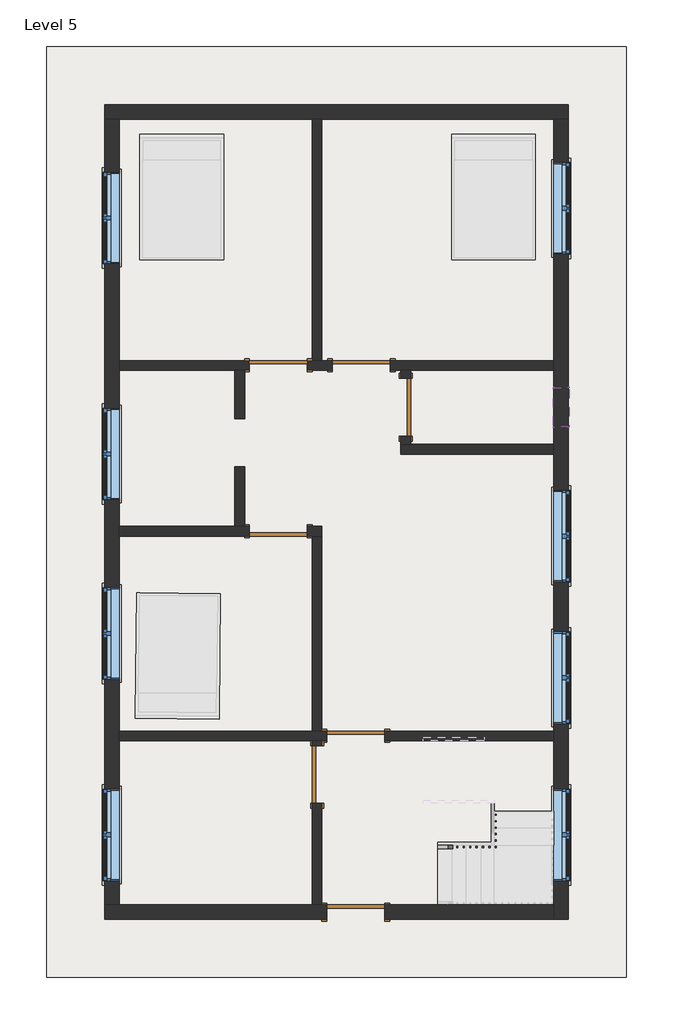
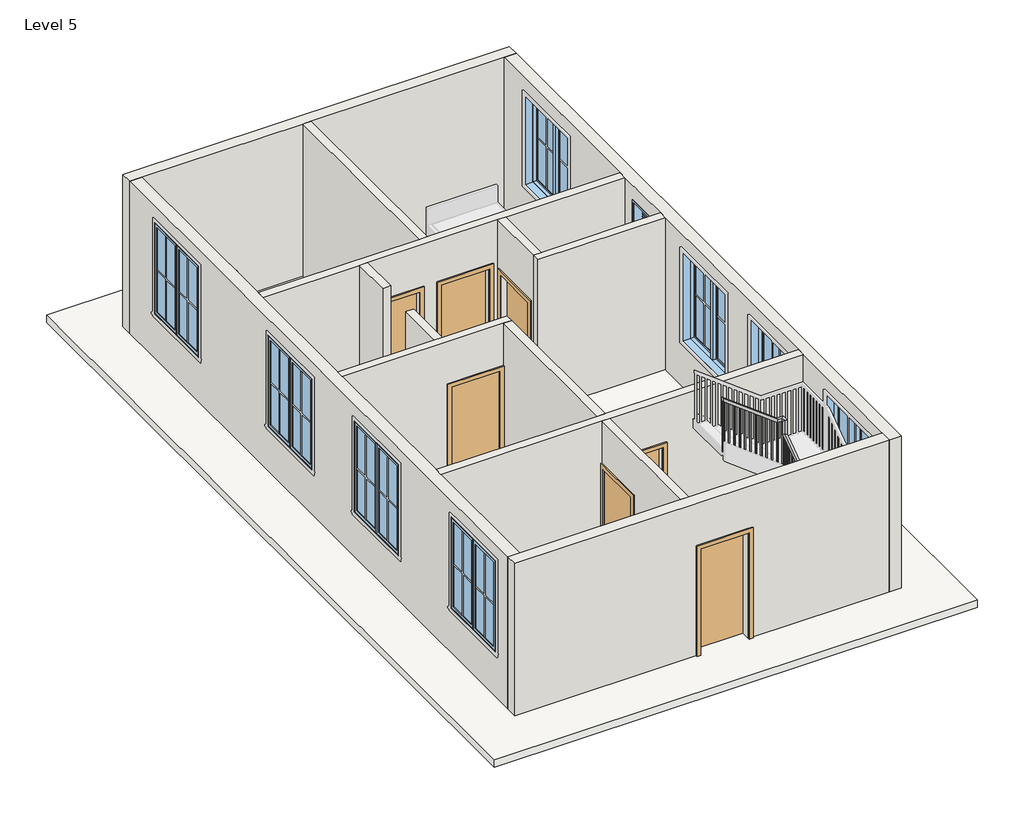
# One storey, part 1 of 2: 14 walls, 9 windows, 7 doors, 1 railing, 1 roof.
"""IFC4 building model written with IfcOpenShell, lengths in millimetres."""

from ifc_helpers import new_model, si_unit, frame, origin, place, context, project, spatial, polyline, outline, extrude, faceted_brep, transform, mapped, element, save
from components import door_2b0b55a0, door_686f89d2, door_16372e1c, door_a90ba1ad, window_9ac97e1a, window_f2d8fef0

model = new_model("IFC4")

# Units and contexts
model_context = context("Model", 3, world=origin())
ifc_project = project(units=[si_unit("LENGTHUNIT", "METRE", prefix="MILLI")], contexts=[model_context])

# Site, building, storey
site = spatial("IfcSite", under=ifc_project)
building = spatial("IfcBuilding", under=site)
storey = spatial("IfcBuildingStorey", under=building, Name="Level 5", Elevation=9601.2)

# Doors
placement = place(None, origin())
door_shape = door_2b0b55a0(model_context)
element("IfcDoor", 1, ObjectType="Single-Flush : 36\" x 80\"", at=placement, inside=storey, context=model_context, shape_type="MappedRepresentation", body=[
    mapped(door_shape, transform((-163.235885, 1707.4649429, 9601.2), x_axis=(0.0, 1.0, 0.0), y_axis=(-1.0, 0.0, 0.0), z_axis=(0.0, 0.0, 1.0))),
])
door_2_shape = door_686f89d2(model_context)
element("IfcDoor", 2, ObjectType="Single-Flush : 36\" x 84\"", at=placement, inside=storey, context=model_context, shape_type="MappedRepresentation", body=[
    mapped(door_2_shape, transform((-861.735885, 2367.8649429, 9601.2), x_axis=(-1.0, 0.0, 0.0), y_axis=(0.0, -1.0, 0.0), z_axis=(0.0, 0.0, 1.0))),
])
element("IfcDoor", 3, ObjectType="Single-Flush : 36\" x 84\"", at=placement, inside=storey, context=model_context, shape_type="MappedRepresentation", body=[
    mapped(door_2_shape, transform((-2169.835885, -248.3350571, 9601.2), x_axis=(1.0, 0.0, 0.0), y_axis=(0.0, 1.0, 0.0), z_axis=(0.0, 0.0, 1.0))),
])
element("IfcDoor", 4, ObjectType="Single-Flush : 36\" x 84\"", at=placement, inside=storey, context=model_context, shape_type="MappedRepresentation", body=[
    mapped(door_2_shape, transform((-950.635885, -3474.1350571, 9601.2), x_axis=(-1.0, 0.0, 0.0), y_axis=(0.0, -1.0, 0.0), z_axis=(0.0, 0.0, 1.0))),
])
door_3_shape = door_16372e1c(model_context)
element("IfcDoor", 5, ObjectType="Single-Flush : 36\" x 84\"", at=placement, inside=storey, context=model_context, shape_type="MappedRepresentation", body=[
    mapped(door_3_shape, transform((-2169.835885, 2367.8649429, 9601.2), x_axis=(1.0, 0.0, 0.0), y_axis=(0.0, 1.0, 0.0), z_axis=(0.0, 0.0, 1.0))),
])
element("IfcDoor", 6, ObjectType="Single-Flush : 36\" x 84\"", at=placement, inside=storey, context=model_context, shape_type="MappedRepresentation", body=[
    mapped(door_3_shape, transform((-1560.235885, -4083.7350571, 9601.2), x_axis=(0.0, 1.0, 0.0), y_axis=(-1.0, 0.0, 0.0), z_axis=(0.0, 0.0, 1.0))),
])
door_4_shape = door_a90ba1ad(model_context)
element("IfcDoor", 7, ObjectType="Single-Flush : 36\" x 84\"", at=placement, inside=storey, context=model_context, shape_type="MappedRepresentation", body=[
    mapped(door_4_shape, transform((-950.635885, -6255.4350571, 9601.2), x_axis=(-1.0, 0.0, 0.0), y_axis=(0.0, -1.0, 0.0), z_axis=(0.0, 0.0, 1.0))),
])

# Railing
element("IfcRailing", 8, ObjectType="Handrail - Rectangular", at=placement, inside=storey, context=model_context, shape_type="SolidModel", body=[
    faceted_brep([(344.764115, -5201.3350571, 10684.9333333), (344.764115, -5201.3350571, 10621.0686436), (344.764115, -5252.1350571, 10621.0686436), (344.764115, -5252.1350571, 10684.9333333), (1157.564115, -5201.3350571, 11304.2095238), (1208.364115, -5201.3350571, 11279.049596), (1208.364115, -5252.1350571, 11279.049596), (1157.564115, -5252.1350571, 11304.2095238), (1157.564115, -5201.3350571, 11586.0285714), (1208.364115, -5201.3350571, 11535.2285714), (1208.364115, -5252.1350571, 11535.2285714), (1157.564115, -5252.1350571, 11586.0285714), (1233.764115, -5201.3350571, 11586.0285714), (1233.764115, -5201.3350571, 11535.2285714), (1284.564115, -5252.1350571, 11535.2285714), (1284.564115, -5252.1350571, 11586.0285714), (1233.764115, -5125.1350571, 11586.0285714), (1233.764115, -5108.8554323, 11535.2285714), (1284.564115, -5108.8554323, 11535.2285714), (1284.564115, -5125.1350571, 11586.0285714), (1233.764115, -4566.3350571, 11985.1714286), (1233.764115, -4515.5350571, 11959.0288395), (1284.564115, -4515.5350571, 11959.0288395), (1284.564115, -4566.3350571, 11985.1714286), (1233.764115, -4566.3350571, 12266.6606061), (1233.764115, -4515.5350571, 12215.8606061), (1284.564115, -4515.5350571, 12215.8606061), (1284.564115, -4566.3350571, 12266.6606061), (1233.764115, -4490.1350571, 12266.6606061), (1233.764115, -4490.1350571, 12215.8606061), (1284.564115, -4439.3350571, 12215.8606061), (1284.564115, -4439.3350571, 12266.6606061), (1157.564115, -4490.1350571, 12266.6606061), (1140.4943334, -4490.1350571, 12215.8606061), (1140.4943334, -4439.3350571, 12215.8606061), (1157.564115, -4439.3350571, 12266.6606061), (116.164115, -4490.1350571, 13055.6), (116.164115, -4439.3350571, 13055.6), (116.164115, -4439.3350571, 12991.8683472), (116.164115, -4490.1350571, 12991.8683472)], [[[0, 1, 2, 3]], [[1, 0, 4, 5]], [[2, 1, 5, 6]], [[3, 2, 6, 7]], [[0, 3, 7, 4]], [[5, 4, 8, 9]], [[6, 5, 9, 10]], [[7, 6, 10, 11]], [[4, 7, 11, 8]], [[9, 8, 12, 13]], [[10, 9, 13, 14]], [[11, 10, 14, 15]], [[8, 11, 15, 12]], [[13, 12, 16, 17]], [[14, 13, 17, 18]], [[15, 14, 18, 19]], [[12, 15, 19, 16]], [[17, 16, 20, 21]], [[18, 17, 21, 22]], [[19, 18, 22, 23]], [[16, 19, 23, 20]], [[21, 20, 24, 25]], [[22, 21, 25, 26]], [[23, 22, 26, 27]], [[20, 23, 27, 24]], [[25, 24, 28, 29]], [[26, 25, 29, 30]], [[27, 26, 30, 31]], [[24, 27, 31, 28]], [[29, 28, 32, 33]], [[30, 29, 33, 34]], [[31, 30, 34, 35]], [[28, 31, 35, 32]], [[36, 37, 38, 39]], [[33, 32, 36, 39]], [[34, 33, 39, 38]], [[35, 34, 38, 37]], [[32, 35, 37, 36]]]),
    extrude(outline(polyline([(12979.8418321, 132.039115), (11971.8666667, 132.039115), (11971.8666667, 151.089115), (12965.4100139, 151.089115), (12979.8418321, 132.039115)])), frame((0.0, -4474.2600571, 0.0), z_axis=(0.0, 1.0, 0.0), x_axis=(0.0, 0.0, 1.0)), (0.0, 0.0, 1.0), 19.05),
    extrude(outline(polyline([(12902.8721351, 233.639115), (11971.8666667, 233.639115), (11971.8666667, 252.689115), (12888.4403169, 252.689115), (12902.8721351, 233.639115)])), frame((0.0, -4474.2600571, 0.0), z_axis=(0.0, 1.0, 0.0), x_axis=(0.0, 0.0, 1.0)), (0.0, 0.0, 1.0), 19.05),
    extrude(outline(polyline([(12825.9024382, 335.239115), (11971.8666667, 335.239115), (11971.8666667, 354.289115), (12811.47062, 354.289115), (12825.9024382, 335.239115)])), frame((0.0, -4474.2600571, 0.0), z_axis=(0.0, 1.0, 0.0), x_axis=(0.0, 0.0, 1.0)), (0.0, 0.0, 1.0), 19.05),
    extrude(outline(polyline([(12748.9327412, 436.839115), (11802.5333333, 436.839115), (11802.5333333, 455.889115), (12734.500923, 455.889115), (12748.9327412, 436.839115)])), frame((0.0, -4474.2600571, 0.0), z_axis=(0.0, 1.0, 0.0), x_axis=(0.0, 0.0, 1.0)), (0.0, 0.0, 1.0), 19.05),
    extrude(outline(polyline([(12671.9630442, 538.439115), (11802.5333333, 538.439115), (11802.5333333, 557.489115), (12657.531226, 557.489115), (12671.9630442, 538.439115)])), frame((0.0, -4474.2600571, 0.0), z_axis=(0.0, 1.0, 0.0), x_axis=(0.0, 0.0, 1.0)), (0.0, 0.0, 1.0), 19.05),
    extrude(outline(polyline([(12594.9933472, 640.039115), (11633.2, 640.039115), (11633.2, 659.089115), (12580.5615291, 659.089115), (12594.9933472, 640.039115)])), frame((0.0, -4474.2600571, 0.0), z_axis=(0.0, 1.0, 0.0), x_axis=(0.0, 0.0, 1.0)), (0.0, 0.0, 1.0), 19.05),
    extrude(outline(polyline([(12518.0236503, 741.639115), (11633.2, 741.639115), (11633.2, 760.689115), (12503.5918321, 760.689115), (12518.0236503, 741.639115)])), frame((0.0, -4474.2600571, 0.0), z_axis=(0.0, 1.0, 0.0), x_axis=(0.0, 0.0, 1.0)), (0.0, 0.0, 1.0), 19.05),
    extrude(outline(polyline([(12441.0539533, 843.239115), (11463.8666667, 843.239115), (11463.8666667, 862.289115), (12426.6221351, 862.289115), (12441.0539533, 843.239115)])), frame((0.0, -4474.2600571, 0.0), z_axis=(0.0, 1.0, 0.0), x_axis=(0.0, 0.0, 1.0)), (0.0, 0.0, 1.0), 19.05),
    extrude(outline(polyline([(12364.0842563, 944.839115), (11463.8666667, 944.839115), (11463.8666667, 963.889115), (12349.6524382, 963.889115), (12364.0842563, 944.839115)])), frame((0.0, -4474.2600571, 0.0), z_axis=(0.0, 1.0, 0.0), x_axis=(0.0, 0.0, 1.0)), (0.0, 0.0, 1.0), 19.05),
    extrude(outline(polyline([(12287.1145594, 1046.439115), (11294.5333333, 1046.439115), (11294.5333333, 1065.489115), (12272.6827412, 1065.489115), (12287.1145594, 1046.439115)])), frame((0.0, -4474.2600571, 0.0), z_axis=(0.0, 1.0, 0.0), x_axis=(0.0, 0.0, 1.0)), (0.0, 0.0, 1.0), 19.05),
    extrude(outline(polyline([(12210.1448624, 1148.039115), (11294.5333333, 1148.039115), (11294.5333333, 1167.089115), (12195.7130442, 1167.089115), (12210.1448624, 1148.039115)])), frame((0.0, -4474.2600571, 0.0), z_axis=(0.0, 1.0, 0.0), x_axis=(0.0, 0.0, 1.0)), (0.0, 0.0, 1.0), 19.05),
    extrude(outline(polyline([(1249.639115, -4525.0600571), (1249.639115, -4506.0100571), (1268.689115, -4506.0100571), (1268.689115, -4525.0600571), (1249.639115, -4525.0600571)])), frame((0.0, 0.0, 10955.8666667), z_axis=(0.0, 0.0, 1.0), x_axis=(1.0, 0.0, 0.0)), (0.0, 0.0, 1.0), 1259.9939394),
    extrude(outline(polyline([(-4607.6100571, 11893.2609823), (-4607.6100571, 10955.8666667), (-4626.6600571, 10955.8666667), (-4626.6600571, 11879.6538395), (-4607.6100571, 11893.2609823)])), frame((1249.639115, 0.0, 0.0), z_axis=(1.0, 0.0, 0.0), x_axis=(0.0, 1.0, 0.0)), (0.0, 0.0, 1.0), 19.05),
    extrude(outline(polyline([(-4709.2100571, 11820.6895538), (-4709.2100571, 10786.5333333), (-4728.2600571, 10786.5333333), (-4728.2600571, 11807.0824109), (-4709.2100571, 11820.6895538)])), frame((1249.639115, 0.0, 0.0), z_axis=(1.0, 0.0, 0.0), x_axis=(0.0, 1.0, 0.0)), (0.0, 0.0, 1.0), 19.05),
    extrude(outline(polyline([(-4810.8100571, 11748.1181252), (-4810.8100571, 10786.5333333), (-4829.8600571, 10786.5333333), (-4829.8600571, 11734.5109823), (-4810.8100571, 11748.1181252)])), frame((1249.639115, 0.0, 0.0), z_axis=(1.0, 0.0, 0.0), x_axis=(0.0, 1.0, 0.0)), (0.0, 0.0, 1.0), 19.05),
    extrude(outline(polyline([(-4912.4100571, 11675.5466966), (-4912.4100571, 10786.5333333), (-4931.4600571, 10786.5333333), (-4931.4600571, 11661.9395538), (-4912.4100571, 11675.5466966)])), frame((1249.639115, 0.0, 0.0), z_axis=(1.0, 0.0, 0.0), x_axis=(0.0, 1.0, 0.0)), (0.0, 0.0, 1.0), 19.05),
    extrude(outline(polyline([(-5014.0100571, 11602.9752681), (-5014.0100571, 10617.2), (-5033.0600571, 10617.2), (-5033.0600571, 11589.3681252), (-5014.0100571, 11602.9752681)])), frame((1249.639115, 0.0, 0.0), z_axis=(1.0, 0.0, 0.0), x_axis=(0.0, 1.0, 0.0)), (0.0, 0.0, 1.0), 19.05),
    extrude(outline(polyline([(-5115.6100571, 11530.4038395), (-5115.6100571, 10617.2), (-5134.6600571, 10617.2), (-5134.6600571, 11516.7966966), (-5115.6100571, 11530.4038395)])), frame((1249.639115, 0.0, 0.0), z_axis=(1.0, 0.0, 0.0), x_axis=(0.0, 1.0, 0.0)), (0.0, 0.0, 1.0), 19.05),
    extrude(outline(polyline([(11233.0876912, 1148.039115), (10278.5333333, 1148.039115), (10278.5333333, 1167.089115), (11247.6019769, 1167.089115), (11233.0876912, 1148.039115)])), frame((0.0, -5236.2600571, 0.0), z_axis=(0.0, 1.0, 0.0), x_axis=(0.0, 0.0, 1.0)), (0.0, 0.0, 1.0), 19.05),
    extrude(outline(polyline([(11155.6781674, 1046.439115), (10278.5333333, 1046.439115), (10278.5333333, 1065.489115), (11170.1924531, 1065.489115), (11155.6781674, 1046.439115)])), frame((0.0, -5236.2600571, 0.0), z_axis=(0.0, 1.0, 0.0), x_axis=(0.0, 0.0, 1.0)), (0.0, 0.0, 1.0), 19.05),
    extrude(outline(polyline([(11078.2686436, 944.839115), (10109.2, 944.839115), (10109.2, 963.889115), (11092.7829293, 963.889115), (11078.2686436, 944.839115)])), frame((0.0, -5236.2600571, 0.0), z_axis=(0.0, 1.0, 0.0), x_axis=(0.0, 0.0, 1.0)), (0.0, 0.0, 1.0), 19.05),
    extrude(outline(polyline([(11000.8591198, 843.239115), (10109.2, 843.239115), (10109.2, 862.289115), (11015.3734055, 862.289115), (11000.8591198, 843.239115)])), frame((0.0, -5236.2600571, 0.0), z_axis=(0.0, 1.0, 0.0), x_axis=(0.0, 0.0, 1.0)), (0.0, 0.0, 1.0), 19.05),
    extrude(outline(polyline([(10923.449596, 741.639115), (9939.8666667, 741.639115), (9939.8666667, 760.689115), (10937.9638817, 760.689115), (10923.449596, 741.639115)])), frame((0.0, -5236.2600571, 0.0), z_axis=(0.0, 1.0, 0.0), x_axis=(0.0, 0.0, 1.0)), (0.0, 0.0, 1.0), 19.05),
    extrude(outline(polyline([(10846.0400722, 640.039115), (9939.8666667, 640.039115), (9939.8666667, 659.089115), (10860.5543579, 659.089115), (10846.0400722, 640.039115)])), frame((0.0, -5236.2600571, 0.0), z_axis=(0.0, 1.0, 0.0), x_axis=(0.0, 0.0, 1.0)), (0.0, 0.0, 1.0), 19.05),
    extrude(outline(polyline([(10768.6305484, 538.439115), (9770.5333333, 538.439115), (9770.5333333, 557.489115), (10783.1448341, 557.489115), (10768.6305484, 538.439115)])), frame((0.0, -5236.2600571, 0.0), z_axis=(0.0, 1.0, 0.0), x_axis=(0.0, 0.0, 1.0)), (0.0, 0.0, 1.0), 19.05),
    extrude(outline(polyline([(10691.2210246, 436.839115), (9770.5333333, 436.839115), (9770.5333333, 455.889115), (10705.7353103, 455.889115), (10691.2210246, 436.839115)])), frame((0.0, -5236.2600571, 0.0), z_axis=(0.0, 1.0, 0.0), x_axis=(0.0, 0.0, 1.0)), (0.0, 0.0, 1.0), 19.05),
    extrude(outline(polyline([(1249.639115, -4474.2600571), (1249.639115, -4455.2100571), (1268.689115, -4455.2100571), (1268.689115, -4474.2600571), (1249.639115, -4474.2600571)])), frame((0.0, 0.0, 11125.2), z_axis=(0.0, 0.0, 1.0), x_axis=(1.0, 0.0, 0.0)), (0.0, 0.0, 1.0), 1090.6606061),
    extrude(outline(polyline([(1249.639115, -5217.2100571), (1268.689115, -5217.2100571), (1268.689115, -5236.2600571), (1249.639115, -5236.2600571), (1249.639115, -5217.2100571)])), frame((0.0, 0.0, 10447.8666667), z_axis=(0.0, 0.0, 1.0), x_axis=(1.0, 0.0, 0.0)), (0.0, 0.0, 1.0), 1087.3619048),
    extrude(outline(polyline([(12991.8683472, 116.164115), (11971.8666667, 116.164115), (11971.8666667, 135.214115), (12977.4365291, 135.214115), (12991.8683472, 116.164115)])), frame((0.0, -4474.2600571, 0.0), z_axis=(0.0, 1.0, 0.0), x_axis=(0.0, 0.0, 1.0)), (0.0, 0.0, 1.0), 19.05),
    extrude(outline(polyline([(10621.0686436, 344.764115), (9770.5333333, 344.764115), (9770.5333333, 363.814115), (10635.5829293, 363.814115), (10621.0686436, 344.764115)])), frame((0.0, -5236.2600571, 0.0), z_axis=(0.0, 1.0, 0.0), x_axis=(0.0, 0.0, 1.0)), (0.0, 0.0, 1.0), 19.05),
])

# Roof
element("IfcRoof", 9, ObjectType="ROOF 6\"", at=placement, inside=storey, context=model_context, shape_type="SweptSolid", body=[
    extrude(outline(polyline([(-5827.435885, 7397.0649429), (3316.564115, 7397.0649429), (3316.564115, -7284.1350571), (-5827.435885, -7284.1350571), (-5827.435885, 7397.0649429)])), frame((0.0, 0.0, 9448.8), z_axis=(0.0, 0.0, 1.0), x_axis=(1.0, 0.0, 0.0)), (0.0, 0.0, 1.0), 152.4),
])

# Walls
element("IfcWall", 10, ObjectType="WALL 6\"", at=placement, inside=storey, context=model_context, shape_type="SweptSolid", body=[
    extrude(outline(polyline([(-1636.435885, 2444.0649429), (-1636.435885, 6254.0649429), (-1484.035885, 6254.0649429), (-1484.035885, 2444.0649429), (-1636.435885, 2444.0649429)])), frame((0.0, 0.0, 9601.2), z_axis=(0.0, 0.0, 1.0), x_axis=(1.0, 0.0, 0.0)), (0.0, 0.0, 1.0), 3048.0),
])
element("IfcWall", 11, ObjectType="WALL 6\"", at=placement, inside=storey, context=model_context, shape_type="Brep", body=[
    faceted_brep([(-1318.935885, 2444.0649429, 9601.2), (-1484.035885, 2444.0649429, 9601.2), (-1636.435885, 2444.0649429, 9601.2), (-1712.635885, 2444.0649429, 9601.2), (-1712.635885, 2444.0649429, 11734.8), (-2627.035885, 2444.0649429, 11734.8), (-2627.035885, 2444.0649429, 9601.2), (-4684.435885, 2444.0649429, 9601.2), (-4684.435885, 2444.0649429, 12649.2), (-1636.435885, 2444.0649429, 12649.2), (-1484.035885, 2444.0649429, 12649.2), (2173.564115, 2444.0649429, 12649.2), (2173.564115, 2444.0649429, 9601.2), (-404.535885, 2444.0649429, 9601.2), (-404.535885, 2444.0649429, 11734.8), (-1318.935885, 2444.0649429, 11734.8), (-1712.635885, 2291.6649429, 11734.8), (-1712.635885, 2291.6649429, 9601.2), (-1318.935885, 2291.6649429, 9601.2), (-1318.935885, 2291.6649429, 11734.8), (-404.535885, 2291.6649429, 11734.8), (-404.535885, 2291.6649429, 9601.2), (-239.435885, 2291.6649429, 9601.2), (-87.035885, 2291.6649429, 9601.2), (2173.564115, 2291.6649429, 9601.2), (2173.564115, 2291.6649429, 12649.2), (-87.035885, 2291.6649429, 12649.2), (-239.435885, 2291.6649429, 12649.2), (-2703.235885, 2291.6649429, 12649.2), (-2855.635885, 2291.6649429, 12649.2), (-4684.435885, 2291.6649429, 12649.2), (-4684.435885, 2291.6649429, 9601.2), (-2855.635885, 2291.6649429, 9601.2), (-2703.235885, 2291.6649429, 9601.2), (-2627.035885, 2291.6649429, 9601.2), (-2627.035885, 2291.6649429, 11734.8)], [[[0, 1, 2, 3, 4, 5, 6, 7, 8, 9, 10, 11, 12, 13, 14, 15]], [[16, 17, 18, 19, 20, 21, 22, 23, 24, 25, 26, 27, 28, 29, 30, 31, 32, 33, 34, 35]], [[13, 12, 24, 23, 22, 21]], [[18, 17, 3, 2, 1, 0]], [[34, 33, 32, 31, 7, 6]], [[12, 11, 25, 24]], [[8, 7, 31, 30]], [[19, 18, 0, 15]], [[20, 19, 15, 14]], [[21, 20, 14, 13]], [[4, 3, 17, 16]], [[5, 4, 16, 35]], [[6, 5, 35, 34]], [[11, 10, 9, 8, 30, 29, 28, 27, 26, 25]]]),
])
element("IfcWall", 12, ObjectType="WALL 6\"", at=placement, inside=storey, context=model_context, shape_type="SweptSolid", body=[
    extrude(outline(polyline([(-2855.635885, 1529.6649429), (-2855.635885, 2291.6649429), (-2703.235885, 2291.6649429), (-2703.235885, 1529.6649429), (-2855.635885, 1529.6649429)])), frame((0.0, 0.0, 9601.2), z_axis=(0.0, 0.0, 1.0), x_axis=(1.0, 0.0, 0.0)), (0.0, 0.0, 1.0), 3048.0),
])
element("IfcWall", 13, ObjectType="WALL 6\"", at=placement, inside=storey, context=model_context, shape_type="Brep", body=[
    faceted_brep([(-1712.635885, -324.5350571, 11734.8), (-1712.635885, -324.5350571, 9601.2), (-1636.435885, -324.5350571, 9601.2), (-1484.035885, -324.5350571, 9601.2), (-1484.035885, -324.5350571, 12649.2), (-1636.435885, -324.5350571, 12649.2), (-4684.435885, -324.5350571, 12649.2), (-4684.435885, -324.5350571, 9601.2), (-2627.035885, -324.5350571, 9601.2), (-2627.035885, -324.5350571, 11734.8), (-1484.035885, -172.1350571, 9601.2), (-1712.635885, -172.1350571, 9601.2), (-1712.635885, -172.1350571, 11734.8), (-2627.035885, -172.1350571, 11734.8), (-2627.035885, -172.1350571, 9601.2), (-2703.235885, -172.1350571, 9601.2), (-2855.635885, -172.1350571, 9601.2), (-4684.435885, -172.1350571, 9601.2), (-4684.435885, -172.1350571, 12649.2), (-2855.635885, -172.1350571, 12649.2), (-2703.235885, -172.1350571, 12649.2), (-1484.035885, -172.1350571, 12649.2)], [[[0, 1, 2, 3, 4, 5, 6, 7, 8, 9]], [[10, 11, 12, 13, 14, 15, 16, 17, 18, 19, 20, 21]], [[8, 7, 17, 16, 15, 14]], [[3, 2, 1, 11, 10]], [[7, 6, 18, 17]], [[4, 3, 10, 21]], [[12, 11, 1, 0]], [[13, 12, 0, 9]], [[14, 13, 9, 8]], [[6, 5, 4, 21, 20, 19, 18]]]),
])
element("IfcWall", 14, ObjectType="WALL 6\"", at=placement, inside=storey, context=model_context, shape_type="SweptSolid", body=[
    extrude(outline(polyline([(-1636.435885, -3397.9350571), (-1636.435885, -324.5350571), (-1484.035885, -324.5350571), (-1484.035885, -3397.9350571), (-1636.435885, -3397.9350571)])), frame((0.0, 0.0, 9601.2), z_axis=(0.0, 0.0, 1.0), x_axis=(1.0, 0.0, 0.0)), (0.0, 0.0, 1.0), 3048.0),
])
element("IfcWall", 15, ObjectType="WALL 6\"", at=placement, inside=storey, context=model_context, shape_type="Brep", body=[
    faceted_brep([(-4684.435885, -3550.3350571, 9601.2), (-1636.435885, -3550.3350571, 9601.2), (-1484.035885, -3550.3350571, 9601.2), (-1407.835885, -3550.3350571, 9601.2), (-1407.835885, -3550.3350571, 11734.8), (-493.435885, -3550.3350571, 11734.8), (-493.435885, -3550.3350571, 9601.2), (2173.564115, -3550.3350571, 9601.2), (2173.564115, -3550.3350571, 12649.2), (-1484.035885, -3550.3350571, 12649.2), (-1636.435885, -3550.3350571, 12649.2), (-4684.435885, -3550.3350571, 12649.2), (-1407.835885, -3397.9350571, 11734.8), (-1407.835885, -3397.9350571, 9601.2), (-1484.035885, -3397.9350571, 9601.2), (-1636.435885, -3397.9350571, 9601.2), (-4684.435885, -3397.9350571, 9601.2), (-4684.435885, -3397.9350571, 12649.2), (-1636.435885, -3397.9350571, 12649.2), (-1484.035885, -3397.9350571, 12649.2), (2173.564115, -3397.9350571, 12649.2), (2173.564115, -3397.9350571, 9601.2), (-493.435885, -3397.9350571, 9601.2), (-493.435885, -3397.9350571, 11734.8)], [[[0, 1, 2, 3, 4, 5, 6, 7, 8, 9, 10, 11]], [[12, 13, 14, 15, 16, 17, 18, 19, 20, 21, 22, 23]], [[22, 21, 7, 6]], [[16, 15, 14, 13, 3, 2, 1, 0]], [[8, 7, 21, 20]], [[0, 11, 17, 16]], [[4, 3, 13, 12]], [[5, 4, 12, 23]], [[6, 5, 23, 22]], [[11, 10, 9, 8, 20, 19, 18, 17]]]),
])
element("IfcWall", 16, ObjectType="WALL 6\"", at=placement, inside=storey, context=model_context, shape_type="SweptSolid", body=[
    extrude(outline(polyline([(-3550.3350571, 9601.2), (-3626.5350571, 9601.2), (-3626.5350571, 11734.8), (-4540.9350571, 11734.8), (-4540.9350571, 9601.2), (-6141.1350571, 9601.2), (-6141.1350571, 12649.2), (-3550.3350571, 12649.2), (-3550.3350571, 9601.2)])), frame((-1636.435885, 0.0, 0.0), z_axis=(1.0, 0.0, 0.0), x_axis=(0.0, 1.0, 0.0)), (0.0, 0.0, 1.0), 152.4),
])
element("IfcWall", 17, ObjectType="WALL 6\"", at=placement, inside=storey, context=model_context, shape_type="Brep", body=[
    faceted_brep([(2173.564115, 1123.2649429, 9601.2), (-87.035885, 1123.2649429, 9601.2), (-239.435885, 1123.2649429, 9601.2), (-239.435885, 1123.2649429, 12649.2), (-87.035885, 1123.2649429, 12649.2), (2173.564115, 1123.2649429, 12649.2), (2173.564115, 970.8649429, 9601.2), (2173.564115, 970.8649429, 12649.2), (-239.435885, 970.8649429, 12649.2), (-239.435885, 970.8649429, 9601.2)], [[[0, 1, 2, 3, 4, 5]], [[6, 7, 8, 9]], [[2, 1, 0, 6, 9]], [[0, 5, 7, 6]], [[3, 2, 9, 8]], [[5, 4, 3, 8, 7]]]),
])
element("IfcWall", 18, ObjectType="WALL 6\"", at=placement, inside=storey, context=model_context, shape_type="SweptSolid", body=[
    extrude(outline(polyline([(2291.6649429, 9601.2), (2164.6649429, 9601.2), (2164.6649429, 11633.2), (1250.2649429, 11633.2), (1250.2649429, 9601.2), (1123.2649429, 9601.2), (1123.2649429, 12649.2), (2291.6649429, 12649.2), (2291.6649429, 9601.2)])), frame((-239.435885, 0.0, 0.0), z_axis=(1.0, 0.0, 0.0), x_axis=(0.0, 1.0, 0.0)), (0.0, 0.0, 1.0), 152.4),
])
element("IfcWall", 19, ObjectType="WALL 6\"", at=placement, inside=storey, context=model_context, shape_type="SweptSolid", body=[
    extrude(outline(polyline([(-2855.635885, -172.1350571), (-2855.635885, 767.6649429), (-2703.235885, 767.6649429), (-2703.235885, -172.1350571), (-2855.635885, -172.1350571)])), frame((0.0, 0.0, 9601.2), z_axis=(0.0, 0.0, 1.0), x_axis=(1.0, 0.0, 0.0)), (0.0, 0.0, 1.0), 3048.0),
])
element("IfcWall", 20, ObjectType="WALL 9\"", at=placement, inside=storey, context=model_context, shape_type="Brep", body=[
    faceted_brep([(-4913.035885, 6254.0649429, 9601.2), (-4684.435885, 6254.0649429, 9601.2), (-1636.435885, 6254.0649429, 9601.2), (-1484.035885, 6254.0649429, 9601.2), (2173.564115, 6254.0649429, 9601.2), (2402.164115, 6254.0649429, 9601.2), (2402.164115, 6254.0649429, 12649.2), (2173.564115, 6254.0649429, 12649.2), (-1484.035885, 6254.0649429, 12649.2), (-1636.435885, 6254.0649429, 12649.2), (-4684.435885, 6254.0649429, 12649.2), (-4913.035885, 6254.0649429, 12649.2), (-4913.035885, 6482.6649429, 9601.2), (-4913.035885, 6482.6649429, 12649.2), (2402.164115, 6482.6649429, 12649.2), (2402.164115, 6482.6649429, 9601.2)], [[[0, 1, 2, 3, 4, 5, 6, 7, 8, 9, 10, 11]], [[12, 13, 14, 15]], [[5, 4, 3, 2, 1, 0, 12, 15]], [[6, 5, 15, 14]], [[0, 11, 13, 12]], [[11, 10, 9, 8, 7, 6, 14, 13]]]),
])
element("IfcWall", 21, ObjectType="WALL 9\"", at=placement, inside=storey, context=model_context, shape_type="Brep", body=[
    faceted_brep([(2173.564115, 6254.0649429, 9601.2), (2173.564115, 2444.0649429, 9601.2), (2173.564115, 2291.6649429, 9601.2), (2173.564115, 1123.2649429, 9601.2), (2173.564115, 970.8649429, 9601.2), (2173.564115, -3397.9350571, 9601.2), (2173.564115, -3550.3350571, 9601.2), (2173.564115, -6141.1350571, 9601.2), (2173.564115, -6369.7350571, 9601.2), (2173.564115, -6369.7350571, 12649.2), (2173.564115, -6141.1350571, 12649.2), (2173.564115, -3550.3350571, 12649.2), (2173.564115, -3397.9350571, 12649.2), (2173.564115, 970.8649429, 12649.2), (2173.564115, 1123.2649429, 12649.2), (2173.564115, 2291.6649429, 12649.2), (2173.564115, 2444.0649429, 12649.2), (2173.564115, 6254.0649429, 12649.2), (2173.564115, -5760.1350571, 12344.4), (2173.564115, -5760.1350571, 10515.6), (2173.564115, -4312.3350571, 10515.6), (2173.564115, -4312.3350571, 12344.4), (2173.564115, -3283.6350571, 12344.4), (2173.564115, -3283.6350571, 10515.6), (2173.564115, -1835.8350571, 10515.6), (2173.564115, -1835.8350571, 12344.4), (2173.564115, -1048.4350571, 12344.4), (2173.564115, -1048.4350571, 10515.6), (2173.564115, 399.3649429, 10515.6), (2173.564115, 399.3649429, 12344.4), (2173.564115, 4120.4649429, 12344.4), (2173.564115, 4120.4649429, 10515.6), (2173.564115, 5568.2649429, 10515.6), (2173.564115, 5568.2649429, 12344.4), (2173.564115, 2012.2649429, 12344.4), (2173.564115, 1402.6649429, 12344.4), (2173.564115, 1402.6649429, 11734.8), (2173.564115, 2012.2649429, 11734.8), (2402.164115, 6254.0649429, 9601.2), (2402.164115, 6254.0649429, 12649.2), (2402.164115, -6369.7350571, 12649.2), (2402.164115, -6369.7350571, 9601.2), (2402.164115, -5760.1350571, 12344.4), (2402.164115, -4312.3350571, 12344.4), (2402.164115, -4312.3350571, 10515.6), (2402.164115, -5760.1350571, 10515.6), (2402.164115, -3283.6350571, 12344.4), (2402.164115, -1835.8350571, 12344.4), (2402.164115, -1835.8350571, 10515.6), (2402.164115, -3283.6350571, 10515.6), (2402.164115, -1048.4350571, 12344.4), (2402.164115, 399.3649429, 12344.4), (2402.164115, 399.3649429, 10515.6), (2402.164115, -1048.4350571, 10515.6), (2402.164115, 4120.4649429, 12344.4), (2402.164115, 5568.2649429, 12344.4), (2402.164115, 5568.2649429, 10515.6), (2402.164115, 4120.4649429, 10515.6), (2402.164115, 2012.2649429, 12344.4), (2402.164115, 2012.2649429, 11734.8), (2402.164115, 1402.6649429, 11734.8), (2402.164115, 1402.6649429, 12344.4)], [[[0, 1, 2, 3, 4, 5, 6, 7, 8, 9, 10, 11, 12, 13, 14, 15, 16, 17], [18, 19, 20, 21], [22, 23, 24, 25], [26, 27, 28, 29], [30, 31, 32, 33], [34, 35, 36, 37]], [[38, 39, 40, 41], [42, 43, 44, 45], [46, 47, 48, 49], [50, 51, 52, 53], [54, 55, 56, 57], [58, 59, 60, 61]], [[8, 7, 6, 5, 4, 3, 2, 1, 0, 38, 41]], [[0, 17, 39, 38]], [[9, 8, 41, 40]], [[19, 18, 42, 45]], [[20, 19, 45, 44]], [[21, 20, 44, 43]], [[18, 21, 43, 42]], [[23, 22, 46, 49]], [[24, 23, 49, 48]], [[25, 24, 48, 47]], [[22, 25, 47, 46]], [[27, 26, 50, 53]], [[28, 27, 53, 52]], [[29, 28, 52, 51]], [[26, 29, 51, 50]], [[31, 30, 54, 57]], [[32, 31, 57, 56]], [[33, 32, 56, 55]], [[30, 33, 55, 54]], [[59, 58, 34, 37]], [[60, 59, 37, 36]], [[61, 60, 36, 35]], [[58, 61, 35, 34]], [[17, 16, 15, 14, 13, 12, 11, 10, 9, 40, 39]]]),
])
element("IfcWall", 22, ObjectType="WALL 9\"", at=placement, inside=storey, context=model_context, shape_type="Brep", body=[
    faceted_brep([(-1407.835885, -6141.1350571, 11734.8), (-1407.835885, -6141.1350571, 9601.2), (-1484.035885, -6141.1350571, 9601.2), (-1636.435885, -6141.1350571, 9601.2), (-4684.435885, -6141.1350571, 9601.2), (-4913.035885, -6141.1350571, 9601.2), (-4913.035885, -6141.1350571, 12649.2), (-4684.435885, -6141.1350571, 12649.2), (-1636.435885, -6141.1350571, 12649.2), (-1484.035885, -6141.1350571, 12649.2), (2173.564115, -6141.1350571, 12649.2), (2173.564115, -6141.1350571, 9601.2), (-493.435885, -6141.1350571, 9601.2), (-493.435885, -6141.1350571, 11734.8), (-4913.035885, -6369.7350571, 9601.2), (-1407.835885, -6369.7350571, 9601.2), (-1407.835885, -6369.7350571, 11734.8), (-493.435885, -6369.7350571, 11734.8), (-493.435885, -6369.7350571, 9601.2), (2173.564115, -6369.7350571, 9601.2), (2173.564115, -6369.7350571, 12649.2), (-4913.035885, -6369.7350571, 12649.2)], [[[0, 1, 2, 3, 4, 5, 6, 7, 8, 9, 10, 11, 12, 13]], [[14, 15, 16, 17, 18, 19, 20, 21]], [[12, 11, 19, 18]], [[5, 4, 3, 2, 1, 15, 14]], [[11, 10, 20, 19]], [[6, 5, 14, 21]], [[16, 15, 1, 0]], [[17, 16, 0, 13]], [[18, 17, 13, 12]], [[10, 9, 8, 7, 6, 21, 20]]]),
])
element("IfcWall", 23, ObjectType="WALL 9\"", at=placement, inside=storey, context=model_context, shape_type="Brep", body=[
    faceted_brep([(-4684.435885, -6141.1350571, 9601.2), (-4684.435885, -3550.3350571, 9601.2), (-4684.435885, -3397.9350571, 9601.2), (-4684.435885, -324.5350571, 9601.2), (-4684.435885, -172.1350571, 9601.2), (-4684.435885, 2291.6649429, 9601.2), (-4684.435885, 2444.0649429, 9601.2), (-4684.435885, 6254.0649429, 9601.2), (-4684.435885, 6254.0649429, 12649.2), (-4684.435885, 2444.0649429, 12649.2), (-4684.435885, 2291.6649429, 12649.2), (-4684.435885, -172.1350571, 12649.2), (-4684.435885, -324.5350571, 12649.2), (-4684.435885, -3397.9350571, 12649.2), (-4684.435885, -3550.3350571, 12649.2), (-4684.435885, -6141.1350571, 12649.2), (-4684.435885, -4312.3350571, 12344.4), (-4684.435885, -4312.3350571, 10515.6), (-4684.435885, -5760.1350571, 10515.6), (-4684.435885, -5760.1350571, 12344.4), (-4684.435885, -1137.3350571, 12344.4), (-4684.435885, -1137.3350571, 10515.6), (-4684.435885, -2585.1350571, 10515.6), (-4684.435885, -2585.1350571, 12344.4), (-4684.435885, 1694.7649429, 12344.4), (-4684.435885, 1694.7649429, 10515.6), (-4684.435885, 246.9649429, 10515.6), (-4684.435885, 246.9649429, 12344.4), (-4684.435885, 5415.8649429, 12344.4), (-4684.435885, 5415.8649429, 10515.6), (-4684.435885, 3968.0649429, 10515.6), (-4684.435885, 3968.0649429, 12344.4), (-4913.035885, -6141.1350571, 9601.2), (-4913.035885, -6141.1350571, 12649.2), (-4913.035885, 6254.0649429, 12649.2), (-4913.035885, 6254.0649429, 9601.2), (-4913.035885, -4312.3350571, 12344.4), (-4913.035885, -5760.1350571, 12344.4), (-4913.035885, -5760.1350571, 10515.6), (-4913.035885, -4312.3350571, 10515.6), (-4913.035885, -1137.3350571, 12344.4), (-4913.035885, -2585.1350571, 12344.4), (-4913.035885, -2585.1350571, 10515.6), (-4913.035885, -1137.3350571, 10515.6), (-4913.035885, 1694.7649429, 12344.4), (-4913.035885, 246.9649429, 12344.4), (-4913.035885, 246.9649429, 10515.6), (-4913.035885, 1694.7649429, 10515.6), (-4913.035885, 5415.8649429, 12344.4), (-4913.035885, 3968.0649429, 12344.4), (-4913.035885, 3968.0649429, 10515.6), (-4913.035885, 5415.8649429, 10515.6)], [[[0, 1, 2, 3, 4, 5, 6, 7, 8, 9, 10, 11, 12, 13, 14, 15], [16, 17, 18, 19], [20, 21, 22, 23], [24, 25, 26, 27], [28, 29, 30, 31]], [[32, 33, 34, 35], [36, 37, 38, 39], [40, 41, 42, 43], [44, 45, 46, 47], [48, 49, 50, 51]], [[7, 6, 5, 4, 3, 2, 1, 0, 32, 35]], [[8, 7, 35, 34]], [[0, 15, 33, 32]], [[17, 16, 36, 39]], [[18, 17, 39, 38]], [[19, 18, 38, 37]], [[16, 19, 37, 36]], [[21, 20, 40, 43]], [[22, 21, 43, 42]], [[23, 22, 42, 41]], [[20, 23, 41, 40]], [[25, 24, 44, 47]], [[26, 25, 47, 46]], [[27, 26, 46, 45]], [[24, 27, 45, 44]], [[29, 28, 48, 51]], [[30, 29, 51, 50]], [[31, 30, 50, 49]], [[28, 31, 49, 48]], [[15, 14, 13, 12, 11, 10, 9, 8, 34, 33]]]),
])

# Windows
window_shape = window_9ac97e1a(model_context)
element("IfcWindow", 24, ObjectType="Window-Casement-Double : 57\" x 72\"", at=placement, inside=storey, context=model_context, shape_type="MappedRepresentation", body=[
    mapped(window_shape, transform((-4798.735885, -5036.2350571, 9601.2), x_axis=(0.0, 1.0, 0.0), y_axis=(-1.0, 0.0, 0.0), z_axis=(0.0, 0.0, 1.0))),
])
element("IfcWindow", 25, ObjectType="Window-Casement-Double : 57\" x 72\"", at=placement, inside=storey, context=model_context, shape_type="MappedRepresentation", body=[
    mapped(window_shape, transform((2287.864115, -5036.2350571, 9601.2), x_axis=(0.0, -1.0, 0.0), y_axis=(1.0, 0.0, 0.0), z_axis=(0.0, 0.0, 1.0))),
])
element("IfcWindow", 26, ObjectType="Window-Casement-Double : 57\" x 72\"", at=placement, inside=storey, context=model_context, shape_type="MappedRepresentation", body=[
    mapped(window_shape, transform((2287.864115, -2559.7350571, 9601.2), x_axis=(0.0, -1.0, 0.0), y_axis=(1.0, 0.0, 0.0), z_axis=(0.0, 0.0, 1.0))),
])
element("IfcWindow", 27, ObjectType="Window-Casement-Double : 57\" x 72\"", at=placement, inside=storey, context=model_context, shape_type="MappedRepresentation", body=[
    mapped(window_shape, transform((2287.864115, -324.5350571, 9601.2), x_axis=(0.0, -1.0, 0.0), y_axis=(1.0, 0.0, 0.0), z_axis=(0.0, 0.0, 1.0))),
])
element("IfcWindow", 28, ObjectType="Window-Casement-Double : 57\" x 72\"", at=placement, inside=storey, context=model_context, shape_type="MappedRepresentation", body=[
    mapped(window_shape, transform((-4798.735885, -1861.2350571, 9601.2), x_axis=(0.0, 1.0, 0.0), y_axis=(-1.0, 0.0, 0.0), z_axis=(0.0, 0.0, 1.0))),
])
element("IfcWindow", 29, ObjectType="Window-Casement-Double : 57\" x 72\"", at=placement, inside=storey, context=model_context, shape_type="MappedRepresentation", body=[
    mapped(window_shape, transform((-4798.735885, 970.8649429, 9601.2), x_axis=(0.0, 1.0, 0.0), y_axis=(-1.0, 0.0, 0.0), z_axis=(0.0, 0.0, 1.0))),
])
element("IfcWindow", 30, ObjectType="Window-Casement-Double : 57\" x 72\"", at=placement, inside=storey, context=model_context, shape_type="MappedRepresentation", body=[
    mapped(window_shape, transform((-4798.735885, 4691.9649429, 9601.2), x_axis=(0.0, 1.0, 0.0), y_axis=(-1.0, 0.0, 0.0), z_axis=(0.0, 0.0, 1.0))),
])
element("IfcWindow", 31, ObjectType="Window-Casement-Double : 57\" x 72\"", at=placement, inside=storey, context=model_context, shape_type="MappedRepresentation", body=[
    mapped(window_shape, transform((2287.864115, 4844.3649429, 9601.2), x_axis=(0.0, -1.0, 0.0), y_axis=(1.0, 0.0, 0.0), z_axis=(0.0, 0.0, 1.0))),
])
window_2_shape = window_f2d8fef0(model_context)
element("IfcWindow", 32, ObjectType="Window-Louvers : 24\" x 24\"", at=placement, inside=storey, context=model_context, shape_type="MappedRepresentation", body=[
    mapped(window_2_shape, transform((2294.214115, 1707.4649429, 10820.4), x_axis=(0.0, -1.0, 0.0), y_axis=(1.0, 0.0, 0.0), z_axis=(0.0, 0.0, 1.0))),
])

save(model, "model.ifc")

# Revit data of these elements
# Type "Single-Flush : 36\" x 80\""
#   Type Mark = "6"
#   Construction Type Id = "MDOOR"
#   Assembly Code = "C1020"
#   Analytic Construction = "Metal"
#   Thickness = 0' - 2"
#   Heat Transfer Coefficient (U) = 0.651978 BTU/(h·ft²·°F)
#   Height = 6' - 8"
#   Trim Projection Ext = 0' - 1"
#   Trim Projection Int = 0' - 1"
#   Trim Width = 0' - 3"
#   Width = 3' - 0"
#   Define Thermal Properties by = 1
#   Define Thermal Properties by = 1
#   Door Material = Door - Panel
#   Frame Material = Door - Frame
#   Visual Light Transmittance = 0
#   Solar Heat Gain Coefficient = 0
#   Function = (empty or 0)
#   Wall Closure = (empty or 0)
# Type "Single-Flush : 36\" x 84\""
#   Type Mark = "1"
#   Construction Type Id = "MDOOR"
#   Assembly Code = "C1020"
#   Analytic Construction = "Metal"
#   Thickness = 0' - 2"
#   Heat Transfer Coefficient (U) = 0.651978 BTU/(h·ft²·°F)
#   Height = 7' - 0"
#   Trim Projection Ext = 0' - 1"
#   Trim Projection Int = 0' - 1"
#   Trim Width = 0' - 3"
#   Width = 3' - 0"
#   Define Thermal Properties by = 1
#   Define Thermal Properties by = 1
#   Door Material = Door - Panel
#   Frame Material = Door - Frame
#   Visual Light Transmittance = 0
#   Solar Heat Gain Coefficient = 0
#   Function = (empty or 0)
#   Wall Closure = (empty or 0)
# Type "Handrail - Rectangular"
#   Assembly Code = "C2010400"
#   built-in parameter 1008612 = 0.0416667 (stored number, unit not read)
#   built-in parameter 1008611 = 0.0416667 (stored number, unit not read)
#   built-in parameter 1008609 = 0.333333 (stored number, unit not read)
#   built-in parameter 1008604 = 0.166667 (stored number, unit not read)
#   built-in parameter 1008603 = 0.166667 (stored number, unit not read)
#   Railing Height = 3' - 0"
#   built-in parameter 1008630 = 2
#   built-in parameter 1008610 = 2
#   built-in parameter 1008618 = Baluster - Square : 3/4"
# Type "ROOF 6\""
#   Assembly Code = "B1020"
#   Layers, outside or top first: 0' - 6" no material (function 1)
# Type "WALL 6\""
#   Assembly Code = "B2010"
#   Layers, outside or top first: 0' - 6" no material (function 1)
# Type "WALL 9\""
#   Assembly Code = "B2010"
#   Layers, outside or top first: 0' - 9" no material (function 1)
# Type "Window-Casement-Double : 57\" x 72\""
#   Type Mark = "17"
#   Fire Rating = "0.5h"
#   Assembly Code = "B2020100"
#   Analytic Construction = "Double glazing - domestic"
#   Frame Extension [instance default] = 0' - 0 1/4"
#   Window Inset [instance default] = 0' - 0"
#   Wall Thickness [instance default] = 0' - 6"
#   Interior Wall Closure [instance default] = 0' - 2 1/4"
#   Half Width = 2' - 4 1/2"
#   Visual Light Transmittance = 0.81
#   Thermal Resistance (R) = 1.8146 (h·ft²·°F)/BTU
#   Solar Heat Gain Coefficient = 0.76
#   Rough Width = 4' - 9 1/2"
#   Rough Height = 6' - 0 1/2"
#   Height = 6' - 0"
#   Heat Transfer Coefficient (U) = 0.5511 BTU/(h·ft²·°F)
#   Exterior Wall Closure [instance default] = 0' - 1 1/4"
#   Extension Jamb [instance default] = 0' - 2 1/4"
#   Default Sill Height = 3' - 0"
#   Width = 4' - 9"
#   Define Thermal Properties by = 0
#   Muntin Visibility = yes
#   Interior Trim Visibility [instance default] = yes
#   Exterior Trim Visibility [instance default] = yes
#   Extension Jamb Visibility [instance default] = yes
#   Interior Trim Material = Wood - Stained
#   Muntin Pattern = Muntin Pattern_2x2 : Muntin Pattern_2x2
#   Interior Trim = Trim-Window-Interior-Flat : Picture Frame
#   Interior Frame Material = Wood - Stained
#   Glass Panel Material = Glass
#   Exterior Trim Material = Clad - White
#   Exterior Trim = Trim-Window-Exterior-Flat : with Sill
#   Exterior Frame Material = Clad - White
#   Wall Closure = (empty or 0)
# Type "Window-Louvers : 24\" x 24\""
#   Type Mark = "18"
#   Construction Type Id = "GSP4R"
#   Assembly Code = "B20"
#   Analytic Construction = "1/8 in Pilkington single glazing"
#   Visual Light Transmittance = 0.9
#   Thermal Resistance (R) = 1.53941 (h·ft²·°F)/BTU
#   Solar Heat Gain Coefficient = 0.78
#   Max Height = 1' - 11.74264"
#   Height = 2' - 0"
#   Heat Transfer Coefficient (U) = 0.6496 BTU/(h·ft²·°F)
#   Blade Width [instance default] = 1' - 10 1/2"
#   Blade Vertical Thickness = 0' - 0.35355"
#   Blade Thickness = 0' - 0 1/4"
#   Blade Spacing = 0' - 1 1/2"
#   Blade Height = 0' - 1.85355"
#   Blade Depth = 0' - 3"
#   Blade Angle = 45.00°
#   Default Sill Height = 3' - 0"
#   Trim Projection_Exterior = 0' - 0 1/2"
#   Trim Projection_Interior = 0' - 0 1/2"
#   Trim Width_Exterior = 0' - 1 1/2"
#   Trim Width_Interior = 0' - 1 1/2"
#   Width = 2' - 0"
#   Max Blade Count = 12
#   Define Thermal Properties by = 1
#   Blade Count = 12
#   Frame Material = Birch
#   Louver Material = Birch
#   Trim Exterior Material = Birch
#   Trim Interior Material = Birch
#   Wall Closure = (empty or 0)
# Element 1 (IfcDoor, "Single-Flush : 36\" x 80\"")
#   Phase Created = New Construction
#   Materials on its faces: "Door - Frame", "Door - Panel"
# Elements 2, 3, 4, 5, 6, 7 (IfcDoor, "Single-Flush : 36\" x 84\"")
#   Phase Created = New Construction
#   Materials on its faces: "Door - Frame", "Door - Panel"
# Element 8 (IfcRailing, "Handrail - Rectangular")
#   Phase Created = New Construction
# Element 9 (IfcRoof, "ROOF 6\"")
#   built-in parameter 1001705 = 31.5 (stored number, unit not read)
#   built-in parameter 1001701 = -0.5 (stored number, unit not read)
#   built-in parameter 1001710 = 33615
#   Phase Created = New Construction
#   Materials on its faces: "Default Roof", "Door - Panel"
# Elements 10, 11, 12, 13, 14, 15, 16, 17, 18, 19 (IfcWall, "WALL 6\"")
#   Top Offset = 0' - 0"
#   Base Offset = 0' - 0"
#   Unconnected Height = 10' - 0"
#   wall height = 10' - 0"
#   Phase Created = New Construction
#   Base Constraint = Level 5
#   Materials on its faces: "Default Wall"
# Elements 20, 21, 22, 23 (IfcWall, "WALL 9\"")
#   Top Offset = 0' - 0"
#   Base Offset = 0' - 0"
#   Unconnected Height = 10' - 0"
#   wall height = 10' - 0"
#   Phase Created = New Construction
#   Base Constraint = Level 5
#   Materials on its faces: "Default Wall", "Cherry"
# Element 24 (IfcWindow, "Window-Casement-Double : 57\" x 72\"")
#   Mark = "28"
#   Window Inset = 0' - 0"
#   Interior Wall Closure = 0' - 2 1/4"
#   Frame Extension = 0' - 0 1/4"
#   Exterior Wall Closure = 0' - 1 1/4"
#   Interior Trim Visibility = yes
#   Exterior Trim Visibility = yes
#   Phase Created = New Construction
#   Materials on its faces: "Wood - Stained", "Glass", "Clad - White"
# Element 25 (IfcWindow, "Window-Casement-Double : 57\" x 72\"")
#   Mark = "29"
#   Window Inset = 0' - 0"
#   Interior Wall Closure = 0' - 2 1/4"
#   Frame Extension = 0' - 0 1/4"
#   Exterior Wall Closure = 0' - 1 1/4"
#   Interior Trim Visibility = yes
#   Exterior Trim Visibility = yes
#   Phase Created = New Construction
#   Materials on its faces: "Wood - Stained", "Glass", "Clad - White"
# Element 26 (IfcWindow, "Window-Casement-Double : 57\" x 72\"")
#   Mark = "30"
#   Window Inset = 0' - 0"
#   Interior Wall Closure = 0' - 2 1/4"
#   Frame Extension = 0' - 0 1/4"
#   Exterior Wall Closure = 0' - 1 1/4"
#   Interior Trim Visibility = yes
#   Exterior Trim Visibility = yes
#   Phase Created = New Construction
#   Materials on its faces: "Wood - Stained", "Glass", "Clad - White"
# Element 27 (IfcWindow, "Window-Casement-Double : 57\" x 72\"")
#   Mark = "31"
#   Window Inset = 0' - 0"
#   Interior Wall Closure = 0' - 2 1/4"
#   Frame Extension = 0' - 0 1/4"
#   Exterior Wall Closure = 0' - 1 1/4"
#   Interior Trim Visibility = yes
#   Exterior Trim Visibility = yes
#   Phase Created = New Construction
#   Materials on its faces: "Wood - Stained", "Glass", "Clad - White"
# Element 28 (IfcWindow, "Window-Casement-Double : 57\" x 72\"")
#   Mark = "32"
#   Window Inset = 0' - 0"
#   Interior Wall Closure = 0' - 2 1/4"
#   Frame Extension = 0' - 0 1/4"
#   Exterior Wall Closure = 0' - 1 1/4"
#   Interior Trim Visibility = yes
#   Exterior Trim Visibility = yes
#   Phase Created = New Construction
#   Materials on its faces: "Wood - Stained", "Glass", "Clad - White"
# Element 29 (IfcWindow, "Window-Casement-Double : 57\" x 72\"")
#   Mark = "33"
#   Window Inset = 0' - 0"
#   Interior Wall Closure = 0' - 2 1/4"
#   Frame Extension = 0' - 0 1/4"
#   Exterior Wall Closure = 0' - 1 1/4"
#   Interior Trim Visibility = yes
#   Exterior Trim Visibility = yes
#   Phase Created = New Construction
#   Materials on its faces: "Wood - Stained", "Glass", "Clad - White"
# Element 30 (IfcWindow, "Window-Casement-Double : 57\" x 72\"")
#   Mark = "34"
#   Window Inset = 0' - 0"
#   Interior Wall Closure = 0' - 2 1/4"
#   Frame Extension = 0' - 0 1/4"
#   Exterior Wall Closure = 0' - 1 1/4"
#   Interior Trim Visibility = yes
#   Exterior Trim Visibility = yes
#   Phase Created = New Construction
#   Materials on its faces: "Wood - Stained", "Glass", "Clad - White"
# Element 31 (IfcWindow, "Window-Casement-Double : 57\" x 72\"")
#   Mark = "35"
#   Window Inset = 0' - 0"
#   Interior Wall Closure = 0' - 2 1/4"
#   Frame Extension = 0' - 0 1/4"
#   Exterior Wall Closure = 0' - 1 1/4"
#   Interior Trim Visibility = yes
#   Exterior Trim Visibility = yes
#   Phase Created = New Construction
#   Materials on its faces: "Wood - Stained", "Glass", "Clad - White"
# Element 32 (IfcWindow, "Window-Louvers : 24\" x 24\"")
#   Mark = "36"
#   Blade Width = 1' - 10 1/2"
#   Phase Created = New Construction
#   Materials on its faces: "Birch"
# Materials
#   "Door - Panel": class "Wood", colour RGB 210 159 95, transparency 0, Cost = 0
#   "Door - Frame": colour RGB 118 70 51, transparency 0, Cost = 0
#   "Wood - Stained": class "Wood", colour RGB 224 178 126, transparency 0, Cost = 0
#   "Glass": class "Glass", colour RGB 0 128 192, transparency 0.75, Description = "Soda Lime Glass", Cost = 0
#   "Clad - White": class "Wood", colour RGB 242 242 238, transparency 0, Cost = 0
#   "Birch": class "Wood", colour RGB 224 178 126, transparency 0, Description = "Betula Alleghaniensis", Cost = 0
#   "Default Roof": colour RGB 88 101 114, transparency 0, Cost = 0
#   "Default Wall": colour RGB 128 128 128, transparency 0, Cost = 0
#   "Cherry": class "Wood", colour RGB 226 177 128, transparency 0, Description = "Prunus Serotina", Cost = 0
